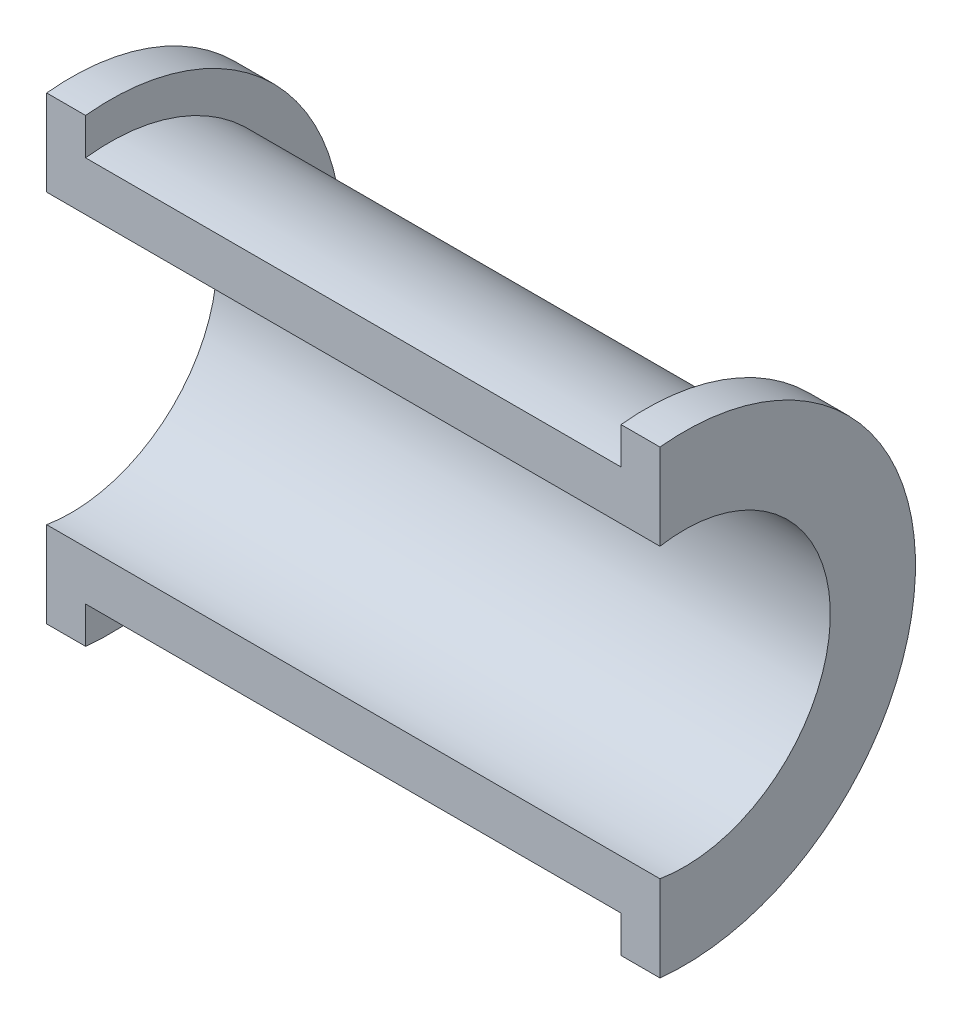
SolidWorks part; units mm, degrees
material "Plain Carbon Steel"
ref_plane "Front Plane" through (0, 0, 0) normal (0, 0, 1) x (1, 0, 0)
ref_plane "Top Plane" through (0, 0, 0) normal (0, 1, 0) x (1, 0, 0)
ref_plane "Right Plane" through (0, 0, 0) normal (1, 0, 0) x (0, 0, -1)
sketch "Half Shell Profile Sketch" plane through (0, 0, 0) normal (1, 0, 0) x (0, 0, -1)
  line L0 (-394.2008, 0) -> (19315.8386, 0) construction
  line L1 (0, -394.2008) -> (0, 19315.8386) construction
  line L2 (0, 39.6863) -> (0, -39.6863)
  arc A0 (0, -39.6863) -> (0, 39.6863) centre (5, 0) ccw
  dimension "D2" = 80
  dimension "D1" = 5
extrude "Half Shell Body" add sketch "Half Shell Profile Sketch" along normal mid plane 110
sketch "End Flange B Sketch Ø95" plane through (55, 0, 0) normal (1, 0, 0) x (0, 0, -1)
  line L0 (0, -1000) -> (0, 49000) construction
  line L1 (0, 47.2361) -> (0, -47.2361)
  arc A0 (0, -47.2361) -> (0, 47.2361) centre (5, 0) ccw
  dimension "D1" = 95
extrude "End Flange B Ø95x8" add sketch "End Flange B Sketch Ø95" along normal blind 8
sketch "End Flange A Sketch Ø95" plane through (-55, 0, 0) normal (-1, 0, 0) x (0, 0, 1)
  line L0 (0, -1000) -> (0, 49000) construction
  line L1 (0, 47.2361) -> (0, -47.2361)
  arc A0 (0, 47.2361) -> (0, -47.2361) centre (-5, 0) ccw
  dimension "D1" = 95
extrude "End Flange A Ø95x8" add sketch "End Flange A Sketch Ø95" along normal blind 8
sketch "Bore Sketch Ø60" plane through (0, 0, 0) normal (1, 0, 0) x (0, 0, -1)
  circle A0 centre (5, 0) radius 30
  dimension "D1" = 60
extrude "Bore Cut Ø60" cut sketch "Bore Sketch Ø60" against normal mid plane 200
